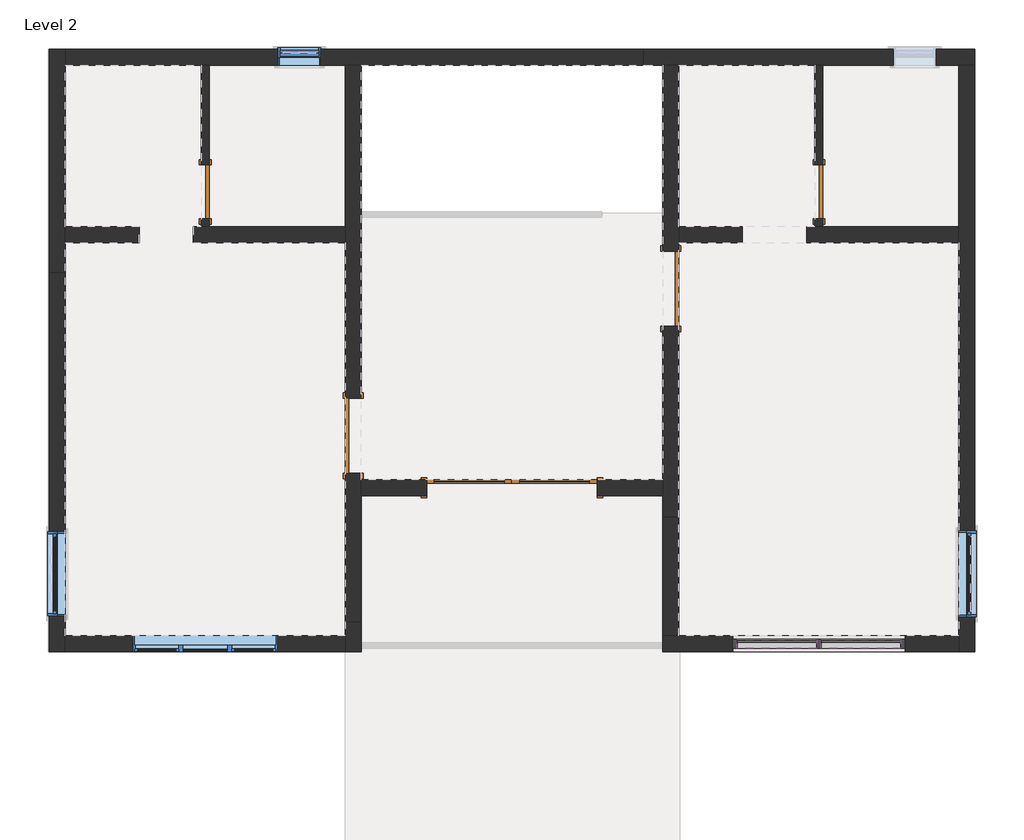
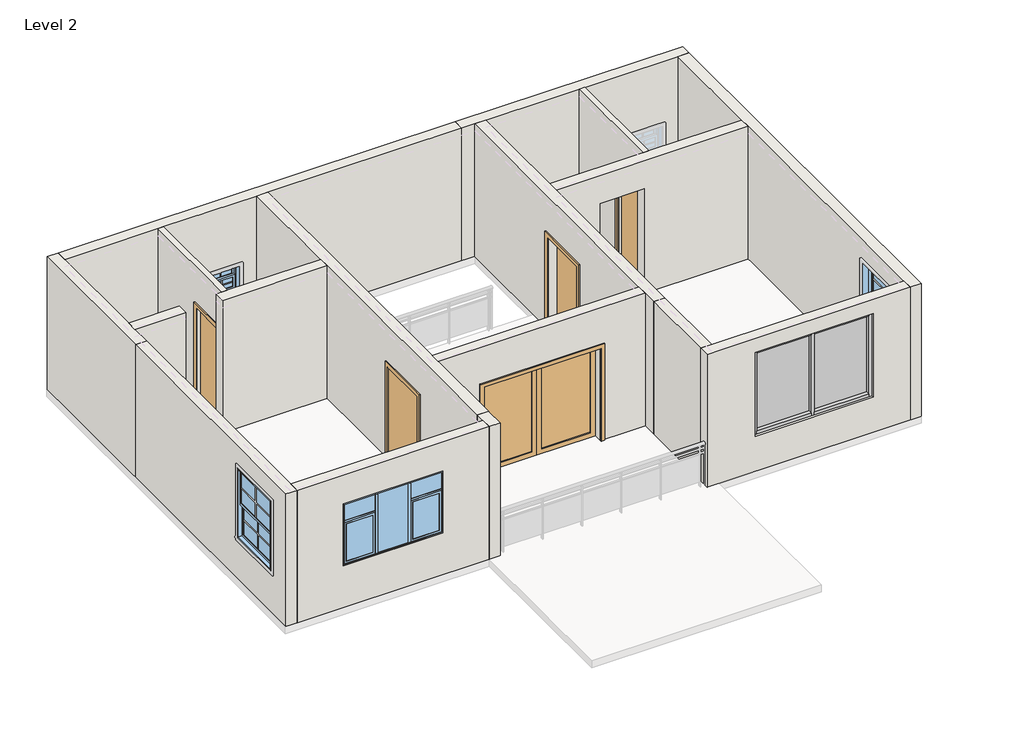
# One storey, part 1 of 2: 17 walls, 7 members, 5 doors, 4 windows, 2 plates.
"""IFC4 building model written with IfcOpenShell, lengths in millimetres."""

from ifc_helpers import new_model, si_unit, frame, origin, place, context, project, spatial, polyline, outline, extrude, faceted_brep, transform, mapped, element, save
from components import door_0e863a58, door_f6232a3f, door_d8f5dbb5, member_d60e8053, member_2fae0574, member_d6c95716, system_panel_glazed_0a36607a, window_casement_triple_side_transom_6_9_71562f8e, window_double_hung_2_x2_15b2d83c, window_double_hung_3_11_b20011b0, window_double_hung_4_x5_5ded1df2

model = new_model("IFC4")

# Units and contexts
model_context = context("Model", 3, world=origin())
ifc_project = project(units=[si_unit("LENGTHUNIT", "METRE", prefix="MILLI")], contexts=[model_context])

# Site, building, storey
site = spatial("IfcSite", under=ifc_project)
building = spatial("IfcBuilding", under=site)
storey = spatial("IfcBuildingStorey", under=building, Name="Level 2", Elevation=3048.0)

# Doors
placement = place(None, origin())
door_shape = door_0e863a58(model_context)
element("IfcDoor", 1, ObjectType="Door-Double-Glass : 7'11\"", at=placement, inside=storey, context=model_context, shape_type="MappedRepresentation", body=[
    mapped(door_shape, transform((-12871.2291129, 5818.4350546, 3048.0), x_axis=(1.0, 0.0, 0.0), y_axis=(0.0, 1.0, 0.0), z_axis=(0.0, 0.0, 1.0))),
])
door_2_shape = door_f6232a3f(model_context)
element("IfcDoor", 2, ObjectType="Single-Flush : 3'6\"", at=placement, inside=storey, context=model_context, shape_type="MappedRepresentation", body=[
    mapped(door_2_shape, transform((-15119.0556236, 6557.4163046, 3048.0), x_axis=(0.0, -1.0, 0.0), y_axis=(1.0, 0.0, 0.0), z_axis=(0.0, 0.0, 1.0))),
])
element("IfcDoor", 3, ObjectType="Single-Flush : 3'6\"", at=placement, inside=storey, context=model_context, shape_type="MappedRepresentation", body=[
    mapped(door_2_shape, transform((-10623.4026022, 8640.2163046, 3048.0), x_axis=(0.0, 1.0, 0.0), y_axis=(-1.0, 0.0, 0.0), z_axis=(0.0, 0.0, 1.0))),
])
door_3_shape = door_d8f5dbb5(model_context)
element("IfcDoor", 4, ObjectType="Single-Flush : 30\" x 80\"", at=placement, inside=storey, context=model_context, shape_type="MappedRepresentation", body=[
    mapped(door_3_shape, transform((-17215.2240665, 10014.1207935, 3048.0), x_axis=(0.0, -1.0, 0.0), y_axis=(1.0, 0.0, 0.0), z_axis=(0.0, 0.0, 1.0))),
])
element("IfcDoor", 5, ObjectType="Single-Flush : 30\" x 80\"", at=placement, inside=storey, context=model_context, shape_type="MappedRepresentation", body=[
    mapped(door_3_shape, transform((-8524.073198, 10013.535577, 3048.0), x_axis=(0.0, -1.0, 0.0), y_axis=(1.0, 0.0, 0.0), z_axis=(0.0, 0.0, 1.0))),
])

# Members
member_shape = member_d60e8053(model_context)
element("IfcMember", 6, ObjectType="Rectangular Mullion : 2.5\" x 5\" rectangular", at=placement, inside=storey, context=model_context, shape_type="MappedRepresentation", body=[
    mapped(member_shape, transform((-8523.3479719, 3612.4962903, 3810.0), x_axis=(1.0, 0.0, 0.0), y_axis=(0.0, -1.0, 0.0), z_axis=(0.0, 0.0, -1.0))),
])
member_2_shape = member_2fae0574(model_context)
element("IfcMember", 7, ObjectType="Rectangular Mullion : 2.5\" x 5\" rectangular", at=placement, inside=storey, context=model_context, shape_type="MappedRepresentation", body=[
    mapped(member_2_shape, transform((-7303.4848741, 3612.4962903, 3810.0), x_axis=(1.0, 0.0, 0.0), y_axis=(0.0, -1.0, 0.0), z_axis=(0.0, 0.0, -1.0))),
])
element("IfcMember", 8, ObjectType="Rectangular Mullion : 2.5\" x 5\" rectangular", at=placement, inside=storey, context=model_context, shape_type="MappedRepresentation", body=[
    mapped(member_2_shape, transform((-9743.2110697, 3612.4962903, 5638.8), x_axis=(-1.0, 0.0, 0.0), y_axis=(0.0, -1.0, 0.0), z_axis=(0.0, 0.0, 1.0))),
])
member_3_shape = member_d6c95716(model_context)
element("IfcMember", 9, ObjectType="Rectangular Mullion : 2.5\" x 5\" rectangular", at=placement, inside=storey, context=model_context, shape_type="MappedRepresentation", body=[
    mapped(member_3_shape, transform((-7366.9848741, 3612.4962903, 5638.8), x_axis=(0.0, 0.0, 1.0), y_axis=(0.0, -1.0, 0.0), z_axis=(1.0, 0.0, 0.0))),
])
element("IfcMember", 10, ObjectType="Rectangular Mullion : 2.5\" x 5\" rectangular", at=placement, inside=storey, context=model_context, shape_type="MappedRepresentation", body=[
    mapped(member_3_shape, transform((-8555.0979719, 3612.4962903, 5638.8), x_axis=(0.0, 0.0, 1.0), y_axis=(0.0, -1.0, 0.0), z_axis=(1.0, 0.0, 0.0))),
])
element("IfcMember", 11, ObjectType="Rectangular Mullion : 2.5\" x 5\" rectangular", at=placement, inside=storey, context=model_context, shape_type="MappedRepresentation", body=[
    mapped(member_3_shape, transform((-9679.7110697, 3612.4962903, 3810.0), x_axis=(0.0, 0.0, -1.0), y_axis=(0.0, -1.0, 0.0), z_axis=(-1.0, 0.0, 0.0))),
])
element("IfcMember", 12, ObjectType="Rectangular Mullion : 2.5\" x 5\" rectangular", at=placement, inside=storey, context=model_context, shape_type="MappedRepresentation", body=[
    mapped(member_3_shape, transform((-8491.5979719, 3612.4962903, 3810.0), x_axis=(0.0, 0.0, -1.0), y_axis=(0.0, -1.0, 0.0), z_axis=(-1.0, 0.0, 0.0))),
])

# Plates
system_panel_glazed_shape = system_panel_glazed_0a36607a(model_context)
element("IfcPlate", 13, ObjectType="System Panel : Glazed", at=placement, inside=storey, context=model_context, shape_type="MappedRepresentation", body=[
    mapped(system_panel_glazed_shape, transform((-9117.4045208, 3612.4962903, 3873.5), x_axis=(1.0, 0.0, 0.0), y_axis=(0.0, 1.0, 0.0), z_axis=(0.0, 0.0, 1.0))),
])
element("IfcPlate", 14, ObjectType="System Panel : Glazed", at=placement, inside=storey, context=model_context, shape_type="MappedRepresentation", body=[
    mapped(system_panel_glazed_shape, transform((-7929.291423, 3612.4962903, 3873.5), x_axis=(1.0, 0.0, 0.0), y_axis=(0.0, 1.0, 0.0), z_axis=(0.0, 0.0, 1.0))),
])

# Walls
element("IfcWall", 15, ObjectType="4.5\"", at=placement, inside=storey, context=model_context, shape_type="SweptSolid", body=[
    extrude(outline(polyline([(9633.1207935, 5080.0), (9633.1207935, 3048.0), (9518.8207935, 3048.0), (9518.8207935, 5943.6), (11804.9957578, 5943.6), (11804.9957578, 3048.0), (10395.1207935, 3048.0), (10395.1207935, 5080.0), (9633.1207935, 5080.0)])), frame((-17272.3740665, 0.0, 0.0), z_axis=(1.0, 0.0, 0.0), x_axis=(0.0, 1.0, 0.0)), (0.0, 0.0, 1.0), 114.3),
])
element("IfcWall", 16, ObjectType="4.5\"", at=placement, inside=storey, context=model_context, shape_type="SweptSolid", body=[
    extrude(outline(polyline([(9632.535577, 5080.0), (9632.535577, 3048.0), (9518.235577, 3048.0), (9518.235577, 5943.6), (11803.4453953, 5943.6), (11803.4453953, 3048.0), (10394.535577, 3048.0), (10394.535577, 5080.0), (9632.535577, 5080.0)])), frame((-8581.223198, 0.0, 0.0), z_axis=(1.0, 0.0, 0.0), x_axis=(0.0, 1.0, 0.0)), (0.0, 0.0, 1.0), 114.3),
])
element("IfcWall", 17, ObjectType="9\"", at=placement, inside=storey, context=model_context, shape_type="Brep", body=[
    faceted_brep([(-19425.7322207, 8869.9954766, 3048.0), (-19425.7322207, 3498.1962903, 3048.0), (-19425.7322207, 3498.1962903, 5943.6), (-19425.7322207, 8869.9954766, 5943.6), (-19425.7322207, 4006.1962903, 5486.4), (-19425.7322207, 4006.1962903, 3962.4), (-19425.7322207, 5199.9962903, 3962.4), (-19425.7322207, 5199.9962903, 5486.4), (-19197.1322207, 8869.9954766, 3048.0), (-19197.1322207, 8869.9954766, 5943.6), (-19197.1322207, 3726.7962903, 5943.6), (-19197.1322207, 3498.1962903, 5943.6), (-19197.1322207, 3498.1962903, 3048.0), (-19197.1322207, 3726.7962903, 3048.0), (-19197.1322207, 4006.1962903, 5486.4), (-19197.1322207, 5199.9962903, 5486.4), (-19197.1322207, 5199.9962903, 3962.4), (-19197.1322207, 4006.1962903, 3962.4)], [[[0, 1, 2, 3], [4, 5, 6, 7]], [[8, 9, 10, 11, 12, 13], [14, 15, 16, 17]], [[1, 0, 8, 13, 12]], [[3, 2, 11, 10, 9]], [[0, 3, 9, 8]], [[2, 1, 12, 11]], [[5, 4, 14, 17]], [[6, 5, 17, 16]], [[7, 6, 16, 15]], [[4, 7, 15, 14]]]),
])
element("IfcWall", 18, ObjectType="9\"", at=placement, inside=storey, context=model_context, shape_type="Brep", body=[
    faceted_brep([(-19425.7322207, 12033.5957578, 3048.0), (-19425.7322207, 8869.9954766, 3048.0), (-19425.7322207, 8869.9954766, 5943.6), (-19425.7322207, 12033.5957578, 5943.6), (-19197.1322207, 12033.5957578, 3048.0), (-19197.1322207, 12033.5957578, 5943.6), (-19197.1322207, 11804.9957578, 5943.6), (-19197.1322207, 9518.8207935, 5943.6), (-19197.1322207, 9290.2207935, 5943.6), (-19197.1322207, 8869.9954766, 5943.6), (-19197.1322207, 8869.9954766, 3048.0), (-19197.1322207, 9290.2207935, 3048.0), (-19197.1322207, 9518.8207935, 3048.0), (-19197.1322207, 11804.9957578, 3048.0)], [[[0, 1, 2, 3]], [[4, 5, 6, 7, 8, 9, 10, 11, 12, 13]], [[1, 0, 4, 13, 12, 11, 10]], [[2, 1, 10, 9]], [[3, 2, 9, 8, 7, 6, 5]], [[0, 3, 5, 4]]]),
])
element("IfcWall", 19, ObjectType="9\"", at=placement, inside=storey, context=model_context, shape_type="Brep", body=[
    faceted_brep([(-11009.5531945, 12033.5957578, 3048.0), (-19197.1322207, 12033.5957578, 3048.0), (-19197.1322207, 12033.5957578, 5943.6), (-11009.5531945, 12033.5957578, 5943.6), (-16185.8556236, 12033.5957578, 4572.0), (-16185.8556236, 12033.5957578, 3962.4), (-15576.2556236, 12033.5957578, 3962.4), (-15576.2556236, 12033.5957578, 4572.0), (-11009.5531945, 11804.9957578, 3048.0), (-11009.5531945, 11804.9957578, 5943.6), (-15004.7556236, 11804.9957578, 5943.6), (-15233.3556236, 11804.9957578, 5943.6), (-17158.0740665, 11804.9957578, 5943.6), (-17272.3740665, 11804.9957578, 5943.6), (-19197.1322207, 11804.9957578, 5943.6), (-19197.1322207, 11804.9957578, 3048.0), (-17272.3740665, 11804.9957578, 3048.0), (-17158.0740665, 11804.9957578, 3048.0), (-15233.3556236, 11804.9957578, 3048.0), (-15004.7556236, 11804.9957578, 3048.0), (-16185.8556236, 11804.9957578, 4572.0), (-15576.2556236, 11804.9957578, 4572.0), (-15576.2556236, 11804.9957578, 3962.4), (-16185.8556236, 11804.9957578, 3962.4)], [[[0, 1, 2, 3], [4, 5, 6, 7]], [[8, 9, 10, 11, 12, 13, 14, 15, 16, 17, 18, 19], [20, 21, 22, 23]], [[1, 0, 8, 19, 18, 17, 16, 15]], [[3, 2, 14, 13, 12, 11, 10, 9]], [[0, 3, 9, 8]], [[2, 1, 15, 14]], [[5, 4, 20, 23]], [[6, 5, 23, 22]], [[7, 6, 22, 21]], [[4, 7, 21, 20]]]),
])
element("IfcWall", 20, ObjectType="9\"", at=placement, inside=storey, context=model_context, shape_type="Brep", body=[
    faceted_brep([(-6315.3817031, 12033.5957578, 3048.0), (-11009.5531945, 12033.5957578, 3048.0), (-11009.5531945, 12033.5957578, 5943.6), (-6315.3817031, 12033.5957578, 5943.6), (-7471.0817031, 12033.5957578, 4572.0), (-7471.0817031, 12033.5957578, 3962.4), (-6861.4817031, 12033.5957578, 3962.4), (-6861.4817031, 12033.5957578, 4572.0), (-6315.3817031, 11804.9957578, 3048.0), (-6315.3817031, 11804.9957578, 5943.6), (-6543.9817031, 11804.9957578, 5943.6), (-10509.1026022, 11804.9957578, 5943.6), (-10737.7026022, 11804.9957578, 5943.6), (-11009.5531945, 11804.9957578, 5943.6), (-11009.5531945, 11804.9957578, 3048.0), (-10737.7026022, 11804.9957578, 3048.0), (-10509.1026022, 11804.9957578, 3048.0), (-6543.9817031, 11804.9957578, 3048.0), (-7471.0817031, 11804.9957578, 4572.0), (-6861.4817031, 11804.9957578, 4572.0), (-6861.4817031, 11804.9957578, 3962.4), (-7471.0817031, 11804.9957578, 3962.4)], [[[0, 1, 2, 3], [4, 5, 6, 7]], [[8, 9, 10, 11, 12, 13, 14, 15, 16, 17], [18, 19, 20, 21]], [[1, 0, 8, 17, 16, 15, 14]], [[2, 1, 14, 13]], [[3, 2, 13, 12, 11, 10, 9]], [[0, 3, 9, 8]], [[5, 4, 18, 21]], [[6, 5, 21, 20]], [[7, 6, 20, 19]], [[4, 7, 19, 18]]]),
])
element("IfcWall", 21, ObjectType="9\"", at=placement, inside=storey, context=model_context, shape_type="Brep", body=[
    faceted_brep([(-6315.3817031, 3498.1962903, 3048.0), (-6315.3817031, 11804.9957578, 3048.0), (-6315.3817031, 11804.9957578, 5943.6), (-6315.3817031, 3498.1962903, 5943.6), (-6315.3817031, 5212.6962903, 5486.4), (-6315.3817031, 5212.6962903, 3962.4), (-6315.3817031, 3993.4962903, 3962.4), (-6315.3817031, 3993.4962903, 5486.4), (-6543.9817031, 3498.1962903, 3048.0), (-6543.9817031, 3498.1962903, 5943.6), (-6543.9817031, 3726.7962903, 5943.6), (-6543.9817031, 9289.635577, 5943.6), (-6543.9817031, 9518.235577, 5943.6), (-6543.9817031, 11804.9957578, 5943.6), (-6543.9817031, 11804.9957578, 3048.0), (-6543.9817031, 9518.235577, 3048.0), (-6543.9817031, 9289.635577, 3048.0), (-6543.9817031, 3726.7962903, 3048.0), (-6543.9817031, 5212.6962903, 5486.4), (-6543.9817031, 3993.4962903, 5486.4), (-6543.9817031, 3993.4962903, 3962.4), (-6543.9817031, 5212.6962903, 3962.4)], [[[0, 1, 2, 3], [4, 5, 6, 7]], [[8, 9, 10, 11, 12, 13, 14, 15, 16, 17], [18, 19, 20, 21]], [[1, 0, 8, 17, 16, 15, 14]], [[3, 2, 13, 12, 11, 10, 9]], [[2, 1, 14, 13]], [[0, 3, 9, 8]], [[5, 4, 18, 21]], [[6, 5, 21, 20]], [[7, 6, 20, 19]], [[4, 7, 19, 18]]]),
])
element("IfcWall", 22, ObjectType="9\"", at=placement, inside=storey, context=model_context, shape_type="Brep", body=[
    faceted_brep([(-10737.7026022, 3498.1962903, 3048.0), (-6543.9817031, 3498.1962903, 3048.0), (-6543.9817031, 3498.1962903, 5943.6), (-10737.7026022, 3498.1962903, 5943.6), (-9743.2110697, 3498.1962903, 3810.0), (-9743.2110697, 3498.1962903, 5638.8), (-7303.4848741, 3498.1962903, 5638.8), (-7303.4848741, 3498.1962903, 3810.0), (-6543.9817031, 3726.7962903, 3048.0), (-10507.7583002, 3726.7962903, 3048.0), (-10736.3583002, 3726.7962903, 3048.0), (-10737.7026022, 3726.7962903, 3048.0), (-10737.7026022, 3726.7962903, 5943.6), (-10736.3583002, 3726.7962903, 5943.6), (-10507.7583002, 3726.7962903, 5943.6), (-6543.9817031, 3726.7962903, 5943.6), (-9743.2110697, 3726.7962903, 5638.8), (-9743.2110697, 3726.7962903, 3810.0), (-7303.4848741, 3726.7962903, 3810.0), (-7303.4848741, 3726.7962903, 5638.8)], [[[0, 1, 2, 3], [4, 5, 6, 7]], [[8, 9, 10, 11, 12, 13, 14, 15], [16, 17, 18, 19]], [[1, 0, 11, 10, 9, 8]], [[3, 2, 15, 14, 13, 12]], [[0, 3, 12, 11]], [[2, 1, 8, 15]], [[4, 17, 16, 5]], [[5, 16, 19, 6]], [[6, 19, 18, 7]], [[17, 4, 7, 18]]]),
])
element("IfcWall", 23, ObjectType="9\"", at=placement, inside=storey, context=model_context, shape_type="Brep", body=[
    faceted_brep([(-10507.7583002, 3726.7962903, 3048.0), (-10507.7583002, 5401.1206207, 3048.0), (-10507.7583002, 5401.1206207, 5943.6), (-10507.7583002, 3726.7962903, 5943.6), (-10736.3583002, 3726.7962903, 3048.0), (-10736.3583002, 3726.7962903, 5943.6), (-10736.3583002, 5401.1206207, 5943.6), (-10736.3583002, 5401.1206207, 3048.0), (-10509.1026022, 5401.1206207, 3048.0), (-10509.1026022, 5401.1206207, 5943.6)], [[[0, 1, 2, 3]], [[4, 5, 6, 7]], [[1, 0, 4, 7, 8]], [[2, 1, 8, 7, 6, 9]], [[3, 2, 9, 6, 5]], [[0, 3, 5, 4]]]),
])
element("IfcWall", 24, ObjectType="9\"", at=placement, inside=storey, context=model_context, shape_type="Brep", body=[
    faceted_brep([(-15233.3556236, 6024.0163046, 5080.0), (-15233.3556236, 6024.0163046, 3048.0), (-15233.3556236, 3917.1170165, 3048.0), (-15233.3556236, 3917.1170165, 5943.6), (-15233.3556236, 9290.2207935, 5943.6), (-15233.3556236, 9518.8207935, 5943.6), (-15233.3556236, 11804.9957578, 5943.6), (-15233.3556236, 11804.9957578, 3048.0), (-15233.3556236, 9518.8207935, 3048.0), (-15233.3556236, 9290.2207935, 3048.0), (-15233.3556236, 7090.8163046, 3048.0), (-15233.3556236, 7090.8163046, 5080.0), (-15004.7556236, 3917.1170165, 3048.0), (-15004.7556236, 5706.5163046, 3048.0), (-15004.7556236, 5935.1163046, 3048.0), (-15004.7556236, 6024.0163046, 3048.0), (-15004.7556236, 6024.0163046, 5080.0), (-15004.7556236, 7090.8163046, 5080.0), (-15004.7556236, 7090.8163046, 3048.0), (-15004.7556236, 11804.9957578, 3048.0), (-15004.7556236, 11804.9957578, 5943.6), (-15004.7556236, 5935.1163046, 5943.6), (-15004.7556236, 5706.5163046, 5943.6), (-15004.7556236, 3917.1170165, 5943.6), (-15005.3951996, 3917.1170165, 3048.0), (-15005.3951996, 3917.1170165, 5943.6)], [[[0, 1, 2, 3, 4, 5, 6, 7, 8, 9, 10, 11]], [[12, 13, 14, 15, 16, 17, 18, 19, 20, 21, 22, 23]], [[2, 1, 15, 14, 13, 12, 24]], [[10, 9, 8, 7, 19, 18]], [[3, 2, 24, 12, 23, 25]], [[6, 5, 4, 3, 25, 23, 22, 21, 20]], [[7, 6, 20, 19]], [[16, 15, 1, 0]], [[17, 16, 0, 11]], [[18, 17, 11, 10]]]),
])
element("IfcWall", 25, ObjectType="9\"", at=placement, inside=storey, context=model_context, shape_type="Brep", body=[
    faceted_brep([(-15005.3951996, 3498.1962903, 3048.0), (-15005.3951996, 3917.1170165, 3048.0), (-15005.3951996, 3917.1170165, 5943.6), (-15005.3951996, 3498.1962903, 5943.6), (-15233.9951996, 3498.1962903, 3048.0), (-15233.9951996, 3498.1962903, 5943.6), (-15233.9951996, 3726.7962903, 5943.6), (-15233.9951996, 3917.1170165, 5943.6), (-15233.9951996, 3917.1170165, 3048.0), (-15233.9951996, 3726.7962903, 3048.0), (-15233.3556236, 3917.1170165, 3048.0), (-15233.3556236, 3917.1170165, 5943.6)], [[[0, 1, 2, 3]], [[4, 5, 6, 7, 8, 9]], [[1, 0, 4, 9, 8, 10]], [[2, 1, 10, 8, 7, 11]], [[3, 2, 11, 7, 6, 5]], [[0, 3, 5, 4]]]),
])
element("IfcWall", 26, ObjectType="9\"", at=placement, inside=storey, context=model_context, shape_type="SweptSolid", body=[
    extrude(outline(polyline([(3048.0, -19197.1322207), (3048.0, -15233.9951996), (5943.6, -15233.9951996), (5943.6, -19197.1322207), (3048.0, -19197.1322207)]), holes=[polyline([(5308.6, -18244.2637102), (5308.6, -16186.8637102), (3962.4, -16186.8637102), (3962.4, -18244.2637102), (5308.6, -18244.2637102)])]), frame((0.0, 3498.1962903, 0.0), z_axis=(0.0, 1.0, 0.0), x_axis=(0.0, 0.0, 1.0)), (0.0, 0.0, 1.0), 228.6),
])
element("IfcWall", 27, ObjectType="9\"", at=placement, inside=storey, context=model_context, shape_type="Brep", body=[
    faceted_brep([(-10737.7026022, 11804.9957578, 3048.0), (-10737.7026022, 9173.6163046, 3048.0), (-10737.7026022, 9173.6163046, 5080.0), (-10737.7026022, 8106.8163046, 5080.0), (-10737.7026022, 8106.8163046, 3048.0), (-10737.7026022, 5935.1163046, 3048.0), (-10737.7026022, 5706.5163046, 3048.0), (-10737.7026022, 5401.1206207, 3048.0), (-10737.7026022, 5401.1206207, 5943.6), (-10737.7026022, 5706.5163046, 5943.6), (-10737.7026022, 5935.1163046, 5943.6), (-10737.7026022, 11804.9957578, 5943.6), (-10509.1026022, 9173.6163046, 5080.0), (-10509.1026022, 9173.6163046, 3048.0), (-10509.1026022, 11804.9957578, 3048.0), (-10509.1026022, 11804.9957578, 5943.6), (-10509.1026022, 5401.1206207, 5943.6), (-10509.1026022, 5401.1206207, 3048.0), (-10509.1026022, 8106.8163046, 3048.0), (-10509.1026022, 8106.8163046, 5080.0), (-10736.3583002, 5401.1206207, 3048.0), (-10736.3583002, 5401.1206207, 5943.6)], [[[0, 1, 2, 3, 4, 5, 6, 7, 8, 9, 10, 11]], [[12, 13, 14, 15, 16, 17, 18, 19]], [[18, 17, 20, 7, 6, 5, 4]], [[14, 13, 1, 0]], [[8, 7, 20, 17, 16, 21]], [[11, 10, 9, 8, 21, 16, 15]], [[0, 11, 15, 14]], [[2, 1, 13, 12]], [[3, 2, 12, 19]], [[4, 3, 19, 18]]]),
])
element("IfcWall", 28, ObjectType="9\"", at=placement, inside=storey, context=model_context, shape_type="SweptSolid", body=[
    extrude(outline(polyline([(-18149.1852461, 9290.2207935), (-19197.1322207, 9290.2207935), (-19197.1322207, 9518.8207935), (-18149.1852461, 9518.8207935), (-18149.1852461, 9290.2207935)])), frame((0.0, 0.0, 3048.0), z_axis=(0.0, 0.0, 1.0), x_axis=(1.0, 0.0, 0.0)), (0.0, 0.0, 1.0), 2895.6),
])
element("IfcWall", 29, ObjectType="9\"", at=placement, inside=storey, context=model_context, shape_type="Brep", body=[
    faceted_brep([(-17388.0183685, 9290.2207935, 3048.0), (-15233.3556236, 9290.2207935, 3048.0), (-15233.3556236, 9290.2207935, 5943.6), (-17388.0183685, 9290.2207935, 5943.6), (-17388.0183685, 9518.8207935, 3048.0), (-17388.0183685, 9518.8207935, 5943.6), (-17272.3740665, 9518.8207935, 5943.6), (-17158.0740665, 9518.8207935, 5943.6), (-15233.3556236, 9518.8207935, 5943.6), (-15233.3556236, 9518.8207935, 3048.0), (-17158.0740665, 9518.8207935, 3048.0), (-17272.3740665, 9518.8207935, 3048.0)], [[[0, 1, 2, 3]], [[4, 5, 6, 7, 8, 9, 10, 11]], [[1, 0, 4, 11, 10, 9]], [[3, 2, 8, 7, 6, 5]], [[0, 3, 5, 4]], [[2, 1, 9, 8]]]),
])
element("IfcWall", 30, ObjectType="9\"", at=placement, inside=storey, context=model_context, shape_type="SweptSolid", body=[
    extrude(outline(polyline([(5080.0, -11664.7291129), (3048.0, -11664.7291129), (3048.0, -10737.7026022), (5943.6, -10737.7026022), (5943.6, -15004.7556236), (3048.0, -15004.7556236), (3048.0, -14077.7291129), (5080.0, -14077.7291129), (5080.0, -11664.7291129)])), frame((0.0, 5706.5163046, 0.0), z_axis=(0.0, 1.0, 0.0), x_axis=(0.0, 0.0, 1.0)), (0.0, 0.0, 1.0), 228.6),
])
element("IfcWall", 31, ObjectType="9\"", at=placement, inside=storey, context=model_context, shape_type="Brep", body=[
    faceted_brep([(-6543.9817031, 9289.635577, 3048.0), (-6543.9817031, 9289.635577, 5943.6), (-10507.0807199, 9289.635577, 5943.6), (-10507.0807199, 9289.635577, 3048.0), (-9606.571224, 9289.635577, 3048.0), (-9606.571224, 9289.635577, 5334.0), (-8694.5162916, 9289.635577, 5334.0), (-8694.5162916, 9289.635577, 3048.0), (-6543.9817031, 9518.235577, 5943.6), (-6543.9817031, 9518.235577, 3048.0), (-8466.923198, 9518.235577, 3048.0), (-8581.223198, 9518.235577, 3048.0), (-8694.5162916, 9518.235577, 3048.0), (-8694.5162916, 9518.235577, 5334.0), (-9606.571224, 9518.235577, 5334.0), (-9606.571224, 9518.235577, 3048.0), (-10507.0807199, 9518.235577, 3048.0), (-10507.0807199, 9518.235577, 5943.6), (-8581.223198, 9518.235577, 5943.6), (-8466.923198, 9518.235577, 5943.6)], [[[0, 1, 2, 3, 4, 5, 6, 7]], [[8, 9, 10, 11, 12, 13, 14, 15, 16, 17, 18, 19]], [[3, 16, 15, 4]], [[9, 0, 7, 12, 11, 10]], [[2, 1, 8, 19, 18, 17]], [[3, 2, 17, 16]], [[1, 0, 9, 8]], [[5, 14, 13, 6]], [[14, 5, 4, 15]], [[6, 13, 12, 7]]]),
])

# Windows
window_casement_triple_side_transom_6_9_shape = window_casement_triple_side_transom_6_9_71562f8e(model_context)
element("IfcWindow", 32, ObjectType="Window-Casement-Triple-Side-Transom : 6'9", at=placement, inside=storey, context=model_context, shape_type="MappedRepresentation", body=[
    mapped(window_casement_triple_side_transom_6_9_shape, transform((-17215.5637102, 3612.4962903, 3048.0), x_axis=(-1.0, 0.0, 0.0), y_axis=(0.0, -1.0, 0.0), z_axis=(0.0, 0.0, 1.0))),
])
window_double_hung_2_x2_shape = window_double_hung_2_x2_15b2d83c(model_context)
element("IfcWindow", 33, ObjectType="Window-Double-Hung : 2'x2'", at=placement, inside=storey, context=model_context, shape_type="MappedRepresentation", body=[
    mapped(window_double_hung_2_x2_shape, transform((-15881.0556236, 11919.2957578, 3048.0), x_axis=(1.0, 0.0, 0.0), y_axis=(0.0, 1.0, 0.0), z_axis=(0.0, 0.0, 1.0))),
])
window_double_hung_3_11_shape = window_double_hung_3_11_b20011b0(model_context)
element("IfcWindow", 34, ObjectType="Window-Double-Hung : 3'11", at=placement, inside=storey, context=model_context, shape_type="MappedRepresentation", body=[
    mapped(window_double_hung_3_11_shape, transform((-19311.4322207, 4603.0962903, 3048.0), x_axis=(0.0, 1.0, 0.0), y_axis=(-1.0, 0.0, 0.0), z_axis=(0.0, 0.0, 1.0))),
])
window_double_hung_4_x5_shape = window_double_hung_4_x5_5ded1df2(model_context)
element("IfcWindow", 35, ObjectType="Window-Double-Hung : 4'x5'", at=placement, inside=storey, context=model_context, shape_type="MappedRepresentation", body=[
    mapped(window_double_hung_4_x5_shape, transform((-6429.6817031, 4603.0962903, 3048.0), x_axis=(0.0, -1.0, 0.0), y_axis=(1.0, 0.0, 0.0), z_axis=(0.0, 0.0, 1.0))),
])

save(model, "model.ifc")

# Revit data of these elements
# Type "Door-Double-Glass : 7'11\""
#   Type Mark = "12"
#   Construction Type Id = "opn-d45"
#   Assembly Code = "C1020"
#   Analytic Construction = "Wood frame, double glass door "
#   W = 3' - 11 1/2"
#   Thickness = 0' - 2"
#   Thermal Resistance (R) = 1.8150 (h·ft²·°F)/BTU
#   Swing Angle [instance default] = 90.00°
#   Heat Transfer Coefficient (U) = 0.5510 BTU/(h·ft²·°F)
#   Height = 6' - 8"
#   Bottom Rail = 0' - 4"
#   Top Rail = 0' - 4"
#   Stiles = 0' - 4"
#   Trim Projection = 0' - 1"
#   Trim Width = 0' - 3"
#   Width = 7' - 11"
#   Define Thermal Properties by = 1
#   Glazing = Glass
#   Panel Material = Wood - Birch - Solid Stained Light Low Gloss
#   Trim Material = Paint - Sienna
#   Visual Light Transmittance = 0
#   Solar Heat Gain Coefficient = 0
#   Function = (empty or 0)
#   Wall Closure = (empty or 0)
# Type "Single-Flush : 3'6\""
#   Type Mark = "11"
#   Construction Type Id = "MDOOR"
#   Assembly Code = "C1020"
#   Analytic Construction = "Metal"
#   Thickness = 0' - 2"
#   Heat Transfer Coefficient (U) = 0.651978 BTU/(h·ft²·°F)
#   Height = 6' - 8"
#   Trim Projection Ext = 0' - 1"
#   Trim Projection Int = 0' - 1"
#   Trim Width = 0' - 3"
#   Width = 3' - 6"
#   Define Thermal Properties by = 1
#   Door Material = Door - Panel
#   Frame Material = Door - Frame
#   Visual Light Transmittance = 0
#   Solar Heat Gain Coefficient = 0
#   Function = (empty or 0)
#   Wall Closure = (empty or 0)
# Type "Single-Flush : 30\" x 80\""
#   Type Mark = "5"
#   Construction Type Id = "MDOOR"
#   Assembly Code = "C1020"
#   Analytic Construction = "Metal"
#   Thickness = 0' - 2"
#   Heat Transfer Coefficient (U) = 0.651978 BTU/(h·ft²·°F)
#   Height = 6' - 8"
#   Trim Projection Ext = 0' - 1"
#   Trim Projection Int = 0' - 1"
#   Trim Width = 0' - 3"
#   Width = 2' - 6"
#   Define Thermal Properties by = 1
#   Define Thermal Properties by = 1
#   Door Material = Door - Panel
#   Frame Material = Door - Frame
#   Visual Light Transmittance = 0
#   Solar Heat Gain Coefficient = 0
#   Function = (empty or 0)
#   Wall Closure = (empty or 0)
# Type "Rectangular Mullion : 2.5\" x 5\" rectangular"
#   built-in parameter 1007304 = 0.416667 (stored number, unit not read)
#   built-in parameter 1007301 = 0.104167 (stored number, unit not read)
#   built-in parameter 1007300 = 0.104167 (stored number, unit not read)
# Type "System Panel : Glazed"
#   Construction Type Id = "GSP4R"
#   Analytic Construction = "1/8 in Pilkington single glazing"
#   Visual Light Transmittance = 0.9
#   Solar Heat Gain Coefficient = 0.86
#   Heat Transfer Coefficient (U) = 1.18115 BTU/(h·ft²·°F)
#   Define Thermal Properties by = 1
# Type "4.5\""
#   Assembly Code = "B2010"
#   Layers, outside or top first: 0' - 4 1/2" no material (function 1)
# Type "9\""
#   Assembly Code = "B2010"
#   Layers, outside or top first: 0' - 9" no material (function 1)
# Type "Window-Casement-Triple-Side-Transom : 6'9"
#   Type Mark = "25"
#   Fire Rating = "0.5h"
#   Assembly Code = "B2020100"
#   Analytic Construction = "Double glazing - domestic"
#   Window Width = 2' - 3"
#   Window Inset [instance default] = 0' - 0 5/8"
#   Wall Thickness [instance default] = 0' - 6"
#   Visual Light Transmittance = 0.81
#   Transom Height Ratio = 0.3
#   Thermal Resistance (R) = 1.8146 (h·ft²·°F)/BTU
#   Solar Heat Gain Coefficient = 0.76
#   Rough Width = 6' - 9 1/2"
#   Rough Height = 4' - 5 1/2"
#   Open Window Height = 3' - 1.1"
#   Heat Transfer Coefficient (U) = 0.5511 BTU/(h·ft²·°F)
#   Height = 4' - 5"
#   Transom Height = 1' - 3.9"
#   Frame Gap 3 [instance default] = 0' - 1 83/128"
#   Frame Gap 2 [instance default] = 0' - 0 5/8"
#   Frame Gap 1 = 0' - 1 51/128"
#   Default Sill Height = 3' - 0"
#   Width = 6' - 9"
#   Frame Material = Metal - Aluminum
#   Glass Panel Material = Glass
#   Wall Closure = (empty or 0)
# Type "Window-Double-Hung : 2'x2'"
#   Type Mark = "26"
#   Fire Rating = "0.5h"
#   Construction Type Id = "DG-DR"
#   Assembly Code = "B2020100"
#   Analytic Construction = "Double glazing - domestic"
#   Wall Thickness [instance default] = 0' - 6"
#   Window Inset [instance default] = 0' - 0"
#   Visual Light Transmittance = 0.81
#   Thermal Resistance (R) = 1.8146 (h·ft²·°F)/BTU
#   Solar Heat Gain Coefficient = 0.76
#   Muntin Width = 1' - 6"
#   Muntin Height = 0' - 8 1/8"
#   Interior Wall Closure [instance default] = 0' - 1 1/2"
#   Rough Width = 2' - 0 1/2"
#   Rough Height = 2' - 0 1/2"
#   Frame Extension [instance default] = 0' - 1 1/4"
#   Exterior Wall Closure [instance default] = 0' - 0 1/2"
#   Extension Jamb [instance default] = 0' - 1 1/2"
#   Heat Transfer Coefficient (U) = 0.5511 BTU/(h·ft²·°F)
#   Height = 2' - 0"
#   Width = 2' - 0"
#   Top Muntin Visibility = yes
#   Indicator Visibility [instance default] = yes
#   Extension Jamb Visibility [instance default] = yes
#   Interior Trim Visibility [instance default] = yes
#   Exterior Trim Visibility [instance default] = yes
#   Define Thermal Properties by = 1
#   Bottom Muntin Visibility = yes
#   Muntin Pattern = Muntin Pattern_2x2 : Muntin Pattern_2x2
#   Interior Trim Material = Wood - Stained
#   Interior Trim = Trim-Window-Interior-Flat : Picture Frame
#   Exterior Trim Material = Clad - White
#   Exterior Trim = Trim-Window-Exterior-Flat : with Sill
#   Glass Panel Material = Glass
#   Exterior Frame Material = Clad - White
#   Interior Frame Material = Wood - Stained
#   Wall Closure = (empty or 0)
# Type "Window-Double-Hung : 3'11"
#   Type Mark = "21"
#   Fire Rating = "0.5h"
#   Construction Type Id = "DG-DR"
#   Assembly Code = "B2020100"
#   Analytic Construction = "Double glazing - domestic"
#   Wall Thickness [instance default] = 0' - 6"
#   Window Inset [instance default] = 0' - 0"
#   Visual Light Transmittance = 0.81
#   Thermal Resistance (R) = 1.8146 (h·ft²·°F)/BTU
#   Solar Heat Gain Coefficient = 0.76
#   Muntin Width = 3' - 5"
#   Muntin Height = 2' - 2 1/8"
#   Interior Wall Closure [instance default] = 0' - 1 1/2"
#   Rough Width = 3' - 11 1/2"
#   Rough Height = 5' - 0 1/2"
#   Frame Extension [instance default] = 0' - 1 1/4"
#   Exterior Wall Closure [instance default] = 0' - 0 1/2"
#   Extension Jamb [instance default] = 0' - 1 1/2"
#   Heat Transfer Coefficient (U) = 0.5511 BTU/(h·ft²·°F)
#   Height = 5' - 0"
#   Width = 3' - 11"
#   Top Muntin Visibility = yes
#   Indicator Visibility [instance default] = yes
#   Extension Jamb Visibility [instance default] = yes
#   Interior Trim Visibility [instance default] = yes
#   Exterior Trim Visibility [instance default] = yes
#   Define Thermal Properties by = 1
#   Bottom Muntin Visibility = yes
#   Muntin Pattern = Muntin Pattern_2x2 : Muntin Pattern_2x2
#   Interior Trim Material = Wood - Stained
#   Interior Trim = Trim-Window-Interior-Flat : Picture Frame
#   Exterior Trim Material = Clad - White
#   Exterior Trim = Trim-Window-Exterior-Flat : with Sill
#   Glass Panel Material = Glass
#   Exterior Frame Material = Clad - White
#   Interior Frame Material = Wood - Stained
#   Wall Closure = (empty or 0)
# Type "Window-Double-Hung : 4'x5'"
#   Type Mark = "27"
#   Fire Rating = "0.5h"
#   Construction Type Id = "DG-DR"
#   Assembly Code = "B2020100"
#   Analytic Construction = "Double glazing - domestic"
#   Wall Thickness [instance default] = 0' - 6"
#   Window Inset [instance default] = 0' - 0"
#   Visual Light Transmittance = 0.81
#   Thermal Resistance (R) = 1.8146 (h·ft²·°F)/BTU
#   Solar Heat Gain Coefficient = 0.76
#   Muntin Width = 3' - 6"
#   Muntin Height = 2' - 2 1/8"
#   Interior Wall Closure [instance default] = 0' - 1 1/2"
#   Rough Width = 4' - 0 1/2"
#   Rough Height = 5' - 0 1/2"
#   Frame Extension [instance default] = 0' - 1 1/4"
#   Exterior Wall Closure [instance default] = 0' - 0 1/2"
#   Extension Jamb [instance default] = 0' - 1 1/2"
#   Heat Transfer Coefficient (U) = 0.5511 BTU/(h·ft²·°F)
#   Height = 5' - 0"
#   Width = 4' - 0"
#   Top Muntin Visibility = yes
#   Indicator Visibility [instance default] = yes
#   Extension Jamb Visibility [instance default] = yes
#   Interior Trim Visibility [instance default] = yes
#   Exterior Trim Visibility [instance default] = yes
#   Define Thermal Properties by = 1
#   Bottom Muntin Visibility = yes
#   Muntin Pattern = Muntin Pattern_2x2 : Muntin Pattern_2x2
#   Interior Trim Material = Wood - Stained
#   Interior Trim = Trim-Window-Interior-Flat : Picture Frame
#   Exterior Trim Material = Clad - White
#   Exterior Trim = Trim-Window-Exterior-Flat : with Sill
#   Glass Panel Material = Glass
#   Exterior Frame Material = Clad - White
#   Interior Frame Material = Wood - Stained
#   Wall Closure = (empty or 0)
# Element 1 (IfcDoor, "Door-Double-Glass : 7'11\"")
#   Swing Angle = 90.00°
#   Phase Created = New Construction
#   Materials on its faces: "Wood - Birch - Solid Stained Light Low Gloss", "Paint - Sienna", "Glass"
# Elements 2, 3 (IfcDoor, "Single-Flush : 3'6\"")
#   Phase Created = New Construction
#   Materials on its faces: "Door - Frame", "Door - Panel"
# Elements 4, 5 (IfcDoor, "Single-Flush : 30\" x 80\"")
#   Phase Created = New Construction
#   Materials on its faces: "Door - Frame", "Door - Panel"
# Elements 6, 7, 8, 9, 10, 11, 12 (IfcMember, "Rectangular Mullion : 2.5\" x 5\" rectangular")
#   Phase Created = New Construction
#   Materials on its faces: "Aluminum"
# Elements 13, 14 (IfcPlate, "System Panel : Glazed")
#   Phase Created = New Construction
#   Materials on its faces: "Glass"
# Elements 15, 16 (IfcWall, "4.5\"")
#   Top Offset = 10' - 0"
#   Base Offset = 0' - 0"
#   wall height = 9' - 6"
#   Phase Created = New Construction
#   Base Constraint = Level 2
#   Top Constraint = 1 slab level
#   Materials on its faces: "Default Wall"
# Elements 17, 18, 19, 20, 21, 22, 23, 24, 25, 26, 27, 28, 29, 30, 31 (IfcWall, "9\"")
#   Top Offset = 10' - 0"
#   Base Offset = 0' - 0"
#   wall height = 9' - 6"
#   Phase Created = New Construction
#   Base Constraint = Level 2
#   Top Constraint = 1 slab level
#   Materials on its faces: "Default Wall"
# Element 32 (IfcWindow, "Window-Casement-Triple-Side-Transom : 6'9")
#   Mark = "15"
#   Window Inset = 0' - 0 5/8"
#   Frame Gap 3 = 0' - 1 83/128"
#   Frame Gap 2 = 0' - 0 5/8"
#   Phase Created = New Construction
#   Materials on its faces: "Metal - Aluminum", "Glass"
# Element 33 (IfcWindow, "Window-Double-Hung : 2'x2'")
#   Mark = "12"
#   Window Inset = 0' - 0"
#   Interior Wall Closure = 0' - 1 1/2"
#   Frame Extension = 0' - 1 1/4"
#   Exterior Wall Closure = 0' - 0 1/2"
#   Interior Trim Visibility = yes
#   Indicator Visibility = yes
#   Exterior Trim Visibility = yes
#   Phase Created = New Construction
#   Materials on its faces: "Wood - Stained", "Glass", "Clad - White"
# Element 34 (IfcWindow, "Window-Double-Hung : 3'11")
#   Mark = "10"
#   Window Inset = 0' - 0"
#   Interior Wall Closure = 0' - 1 1/2"
#   Frame Extension = 0' - 1 1/4"
#   Exterior Wall Closure = 0' - 0 1/2"
#   Interior Trim Visibility = yes
#   Indicator Visibility = yes
#   Exterior Trim Visibility = yes
#   Phase Created = New Construction
#   Materials on its faces: "Wood - Stained", "Glass", "Clad - White"
# Element 35 (IfcWindow, "Window-Double-Hung : 4'x5'")
#   Mark = "11"
#   Window Inset = 0' - 0"
#   Interior Wall Closure = 0' - 1 1/2"
#   Frame Extension = 0' - 1 1/4"
#   Exterior Wall Closure = 0' - 0 1/2"
#   Interior Trim Visibility = yes
#   Indicator Visibility = yes
#   Exterior Trim Visibility = yes
#   Phase Created = New Construction
#   Materials on its faces: "Wood - Stained", "Glass", "Clad - White"
# Materials
#   "Glass": class "Glass", colour RGB 154 182 205, transparency 0.85, Description = "Soda Lime Glass", Cost = 0
#   "Wood - Birch - Solid Stained Light Low Gloss": class "Wood", colour RGB 210 159 95, transparency 0, Cost = 0
#   "Paint - Sienna": colour RGB 118 70 51, transparency 0, Cost = 0
#   "Door - Panel": class "Wood", colour RGB 210 159 95, transparency 0, Cost = 0
#   "Door - Frame": colour RGB 118 70 51, transparency 0, Cost = 0
#   "Metal - Aluminum": class "Metal", colour RGB 247 247 247, transparency 0
#   "Wood - Stained": class "Wood", colour RGB 224 178 126, transparency 0, Cost = 0
#   "Clad - White": class "Wood", colour RGB 242 242 238, transparency 0, Cost = 0
#   "Aluminum": class "Metal", colour RGB 247 247 247, transparency 0, Description = "Aluminum 6061", Cost = 0
#   "Default Wall": colour RGB 128 128 128, transparency 0, Cost = 0
